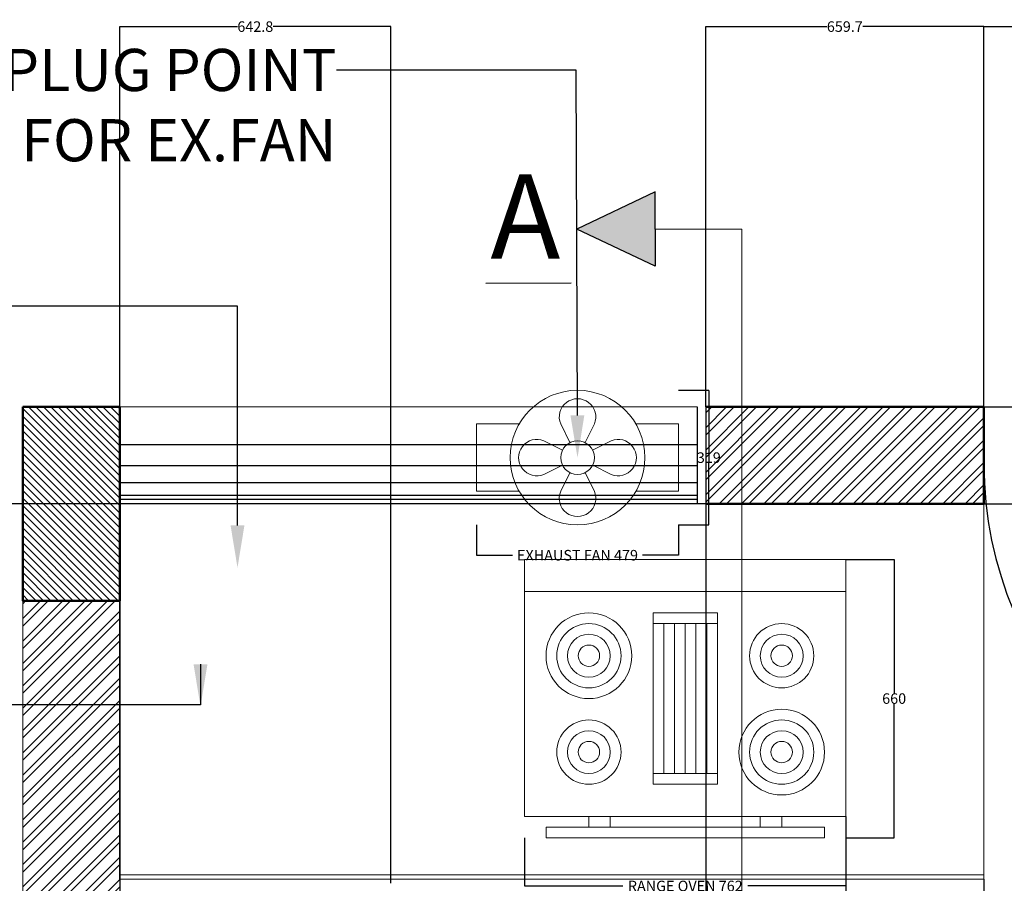
# Model space of a CAD drawing. Units: millimetres. Extents: x 1944 to 29915, y -10550 to 5909.
# Tile 8 of 24: x 6709 to 9044, y 3861 to 5909. Entities that reach past the tile are written whole.
import ezdxf
from ezdxf import colors
from ezdxf.entities.mleader import LeaderData, LeaderLine
from ezdxf.math import Vec2, Vec3

# ---------------------------------------------------------------- set-up
doc = ezdxf.new("R2010")
doc.units = ezdxf.units.MM
doc.header["$MEASUREMENT"] = 0
for name, color, linetype, lineweight in [('A-ANNO-DIMS', 2, 'Continuous', 18), ('A-ANNO-SYMB', 2, 'Continuous', 18), ('A-ANNO-TEXT', 7, 'Continuous', 25), ('A-DOOR', 4, 'Continuous', 25), ('A-EQPM', 6, 'Continuous', 18), ('A-FLOR-FIXT', 9, 'Continuous', 18), ('A-GLAZ', 4, 'Continuous', 25), ('A-WALL', 7, 'Continuous', 50), ('A-WALL-PATT', 8, 'Continuous', 18)]:
    doc.layers.add(name, color=color, linetype=linetype, lineweight=lineweight)
doc.styles.get("Standard").update_dxf_attribs({"font": 'arial.ttf'})
doc.dimstyles.get("Standard").update_dxf_attribs({"dimtxt": 25, "dimasz": 0.18, "dimexe": 0.18, "dimexo": 0.0625, "dimgap": 0.09, "dimtad": 0, "dimtih": 1, "dimtoh": 1, "dimdec": 0, "dimzin": 0, "dimdsep": 46, "dimtxsty": 'Standard', "dimcen": 0.09, "dimadec": 0, "dimazin": 0, "dimtfac": 1, "dimtdec": 0, "dimtofl": 0, "dimtmove": 0, "dimatfit": 3, "dimfxl": 1, "dimtolj": 1, "dimtzin": 0, "dimarcsym": 0})

# ---------------------------------------------------------------- blocks, each defined once
blk = doc.blocks.new('Range-Oven - 30 in top')
for p, q in [((0, -3), (30, -3)), ((12, -6), (18, -6)), ((13, -20), (13, -6)), ((14, -6), (14, -20)), ((15, -20), (15, -6)), ((16, -6), (16, -20)), ((17, -20), (17, -6)), ((18, -20), (12, -20)), ((6, -24), (6, -25)), ((8, -25), (8, -24)), ((22, -25), (22, -24)), ((24, -24), (24, -25))]:
    blk.add_line(p, q)
for points in [[(0, -24), (0, 0), (30, 0), (30, -24)], [(12, -21), (12, -5), (18, -5), (18, -21)], [(2, -26), (2, -25), (28, -25), (28, -26)]]:
    blk.add_lwpolyline(points, close=True)
for centre, radius in [((6, -9), 4), ((6, -9), 3), ((24, -9), 3), ((6, -9), 2), ((24, -9), 2), ((6, -9), 1), ((24, -9), 1), ((24, -18), 4), ((6, -18), 3), ((24, -18), 3), ((6, -18), 2), ((24, -18), 2), ((6, -18), 1), ((24, -18), 1)]:
    blk.add_circle(centre, radius)
blk = doc.blocks.new('Fan')
for p, q in [((0, 0), (0, 0.1)), ((0, 0.1), (0.1287, 0.1)), ((0.2776, 0.0448), (0.25, 0.1)), ((0.35, 0.1), (0.3225, 0.045)), ((0.473, 0.1), (0.6, 0.1)), ((0.6, 0.1), (0.6, 0)), ((0.2552, 0.0224), (0.2, 0.05)), ((0.3448, 0.0224), (0.4, 0.05)), ((0, -0.1), (0, 0)), ((0.6, 0), (0.6, -0.1)), ((0.2, -0.05), (0.255, -0.0225)), ((0.4, -0.05), (0.345, -0.0225)), ((0.2776, -0.0448), (0.25, -0.1)), ((0.35, -0.1), (0.3225, -0.045)), ((0.1278, -0.1), (0, -0.1)), ((0.6, -0.1), (0.4736, -0.1))]:
    blk.add_line(p, q)
blk.add_circle((0.3, 0), 0.05)
for centre, radius, start, end in [((0.3, 0), 0.2, 90, 180), ((0.3, 0), 0.2, 0, 90), ((0.3, 0.1208), 0.0542, 337.3801, 202.6199), ((0.1792, 0), 0.0542, 67.3801, 292.6199), ((0.4208, 0), 0.0542, 247.3801, 112.6199), ((0.3, 0), 0.2, 180, 270), ((0.3, 0), 0.2, 270, 0), ((0.3, -0.1208), 0.0542, 157.3801, 22.6199)]:
    blk.add_arc(centre, radius, start, end)
blk = doc.blocks.new('*U2')
for p, q in [((0, 0), (0, -6)), ((40, 0), (40, -6))]:
    blk.add_line(p, q)
blk.add_lwpolyline([(0, 0), (0, 40), (1.75, 40), (1.75, 0)], close=True)
blk.add_arc((0, 0), 40, 0, 90)
blk = doc.blocks.new('*D38')
at = {"layer": 'A-ANNO-DIMS', "color": 0, "lineweight": -2, "transparency": 16777216}
for p, q in [((7906, 3968.8), (7906, 3854.4)), ((8668, 3968.8), (8668, 3854.4)), ((7906.2, 3854.5), (8138.8, 3854.5)), ((8667.9, 3854.5), (8435.3, 3854.5))]:
    blk.add_line(p, q, dxfattribs=at)
at = {"layer": 'A-ANNO-DIMS', "color": 0, "transparency": 16777216}
for points in [[(7906.2, 3854.6), (7906.2, 3854.5), (7906, 3854.5)], [(8667.9, 3854.6), (8667.9, 3854.5), (8668, 3854.5)]]:
    blk.add_solid(points, dxfattribs=at)
at = {"layer": 'Defpoints', "color": 0, "transparency": 16777216}
for p in [(7906, 3968.8), (8668, 3968.8), (8668, 3854.5)]:
    blk.add_point(p, dxfattribs=at)
at = {"layer": 'A-ANNO-DIMS', "color": 0, "transparency": 16777216, "insert": (8287, 3854.5), "char_height": 25, "attachment_point": 5}
blk.add_mtext('\\A1;RANGE OVEN 762', dxfattribs=at)
blk = doc.blocks.new('*D39')
at = {"layer": 'A-ANNO-DIMS', "color": 0, "lineweight": -2, "transparency": 16777216}
for p, q in [((8668.1, 4629.2), (8782.5, 4629.2)), ((8782.3, 4629.1), (8782.3, 4311.9)), ((8782.3, 3969), (8782.3, 4286.2)), ((8668.1, 3968.8), (8782.5, 3968.8))]:
    blk.add_line(p, q, dxfattribs=at)
at = {"layer": 'A-ANNO-DIMS', "color": 0, "transparency": 16777216}
for points in [[(8782.3, 4629.1), (8782.4, 4629.1), (8782.3, 4629.2)], [(8782.3, 3969), (8782.4, 3969), (8782.3, 3968.8)]]:
    blk.add_solid(points, dxfattribs=at)
at = {"layer": 'Defpoints', "color": 0, "transparency": 16777216}
for p in [(8668, 4629.2), (8782.3, 4629.2), (8668, 3968.8)]:
    blk.add_point(p, dxfattribs=at)
at = {"layer": 'A-ANNO-DIMS', "color": 0, "transparency": 16777216, "insert": (8782.3, 4299), "char_height": 25, "attachment_point": 5}
blk.add_mtext('\\A1;660', dxfattribs=at)
blk = doc.blocks.new('*D44')
at = {"layer": 'A-ANNO-DIMS', "color": 0, "lineweight": -2, "transparency": 16777216}
for p, q in [((7792, 4710.8), (7792, 4638.8)), ((8271, 4710.8), (8271, 4638.8)), ((7792.2, 4639), (7877.3, 4639)), ((8270.8, 4639), (8185.7, 4639))]:
    blk.add_line(p, q, dxfattribs=at)
at = {"layer": 'A-ANNO-DIMS', "color": 0, "transparency": 16777216}
for points in [[(7792.2, 4639), (7792.2, 4638.9), (7792, 4639)], [(8270.8, 4639), (8270.8, 4638.9), (8271, 4639)]]:
    blk.add_solid(points, dxfattribs=at)
at = {"layer": 'Defpoints', "color": 0, "transparency": 16777216}
for p in [(7792, 4710.8), (8271, 4710.8), (8271, 4639)]:
    blk.add_point(p, dxfattribs=at)
at = {"layer": 'A-ANNO-DIMS', "color": 0, "transparency": 16777216, "insert": (8031.5, 4639), "char_height": 25, "attachment_point": 5}
blk.add_mtext('\\A1;EXHAUST FAN 479', dxfattribs=at)
blk = doc.blocks.new('*D45')
at = {"layer": 'A-ANNO-DIMS', "color": 0, "lineweight": -2, "transparency": 16777216}
for p, q in [((8271, 5030.1), (8343, 5030.1)), ((8342.8, 5030), (8342.8, 4883.3)), ((8342.8, 4711), (8342.8, 4857.6)), ((8271, 4710.8), (8343, 4710.8))]:
    blk.add_line(p, q, dxfattribs=at)
at = {"layer": 'A-ANNO-DIMS', "color": 0, "transparency": 16777216}
for points in [[(8342.8, 5030), (8342.9, 5030), (8342.8, 5030.1)], [(8342.8, 4711), (8342.9, 4711), (8342.8, 4710.8)]]:
    blk.add_solid(points, dxfattribs=at)
at = {"layer": 'Defpoints', "color": 0, "transparency": 16777216}
for p in [(8271, 5030.1), (8342.8, 5030.1), (8271, 4710.8)]:
    blk.add_point(p, dxfattribs=at)
at = {"layer": 'A-ANNO-DIMS', "color": 0, "transparency": 16777216, "insert": (8342.8, 4870.5), "char_height": 25, "attachment_point": 5}
blk.add_mtext('\\A1;319', dxfattribs=at)
blk = doc.blocks.new('*D46')
at = {"layer": 'A-ANNO-DIMS', "color": 0, "lineweight": -2, "transparency": 16777216}
for p, q in [((8335.5, 4990.9), (8335.5, 5892.9)), ((8335.7, 5892.8), (8623, 5892.8)), ((8995, 5892.8), (8707.7, 5892.8)), ((8995.2, 4990.9), (8995.2, 5892.9))]:
    blk.add_line(p, q, dxfattribs=at)
at = {"layer": 'A-ANNO-DIMS', "color": 0, "transparency": 16777216}
for points in [[(8335.7, 5892.8), (8335.7, 5892.7), (8335.5, 5892.8)], [(8995, 5892.8), (8995, 5892.7), (8995.2, 5892.8)]]:
    blk.add_solid(points, dxfattribs=at)
at = {"layer": 'Defpoints', "color": 0, "transparency": 16777216}
for p in [(8995.2, 5892.8), (8335.5, 4990.8), (8995.2, 4990.8)]:
    blk.add_point(p, dxfattribs=at)
at = {"layer": 'A-ANNO-DIMS', "color": 0, "transparency": 16777216, "insert": (8665.3, 5892.8), "char_height": 25, "attachment_point": 5}
blk.add_mtext('\\A1;659.7', dxfattribs=at)
blk = doc.blocks.new('*D47')
at = {"layer": 'A-ANNO-DIMS', "color": 0, "lineweight": -2, "transparency": 16777216}
for p, q in [((8995.2, 4990.9), (8995.2, 5892.9)), ((8995.4, 5892.8), (9417.6, 5892.8)), ((9895, 5892.8), (9472.9, 5892.8)), ((9895.2, 4990.9), (9895.2, 5892.9))]:
    blk.add_line(p, q, dxfattribs=at)
at = {"layer": 'A-ANNO-DIMS', "color": 0, "transparency": 16777216}
for points in [[(8995.4, 5892.8), (8995.4, 5892.7), (8995.2, 5892.8)], [(9895, 5892.8), (9895, 5892.7), (9895.2, 5892.8)]]:
    blk.add_solid(points, dxfattribs=at)
at = {"layer": 'Defpoints', "color": 0, "transparency": 16777216}
for p in [(9895.2, 5892.8), (8995.2, 4990.8), (9895.2, 4990.8)]:
    blk.add_point(p, dxfattribs=at)
at = {"layer": 'A-ANNO-DIMS', "color": 0, "transparency": 16777216, "insert": (9445.2, 5892.8), "char_height": 25, "attachment_point": 5}
blk.add_mtext('\\A1;900', dxfattribs=at)
blk = doc.blocks.new('*D49')
at = {"layer": 'A-ANNO-DIMS', "color": 0, "lineweight": -2, "transparency": 16777216}
for p, q in [((8335.5, 4760.8), (8335.5, -697.2)), ((6945.9, 4530.8), (6945.9, -697.2)), ((6946.1, -697), (7589.8, -697)), ((8335.3, -697), (7691.6, -697))]:
    blk.add_line(p, q, dxfattribs=at)
at = {"layer": 'A-ANNO-DIMS', "color": 0, "transparency": 16777216}
for points in [[(6946.1, -697), (6946.1, -697.1), (6945.9, -697)], [(8335.3, -697), (8335.3, -697.1), (8335.5, -697)]]:
    blk.add_solid(points, dxfattribs=at)
at = {"layer": 'Defpoints', "color": 0, "transparency": 16777216}
for p in [(8335.5, 4760.8), (6945.9, 4530.8), (8335.5, -697)]:
    blk.add_point(p, dxfattribs=at)
at = {"layer": 'A-ANNO-DIMS', "color": 0, "transparency": 16777216, "insert": (7640.7, -697), "char_height": 25, "attachment_point": 5}
blk.add_mtext('\\A1;1389.5', dxfattribs=at)
blk = doc.blocks.new('*D55')
at = {"layer": 'A-ANNO-DIMS', "color": 0, "lineweight": -2, "transparency": 16777216}
for p, q in [((8995.3, 4990.8), (11007.7, 4990.8)), ((11007.5, 4990.7), (11007.5, 4888.7)), ((11007.5, 4761), (11007.5, 4863)), ((8995.3, 4760.8), (11007.7, 4760.8))]:
    blk.add_line(p, q, dxfattribs=at)
at = {"layer": 'A-ANNO-DIMS', "color": 0, "transparency": 16777216}
for points in [[(11007.5, 4990.7), (11007.5, 4990.7), (11007.5, 4990.8)], [(11007.5, 4761), (11007.5, 4761), (11007.5, 4760.8)]]:
    blk.add_solid(points, dxfattribs=at)
at = {"layer": 'Defpoints', "color": 0, "transparency": 16777216}
for p in [(8995.2, 4990.8), (8995.2, 4760.8), (11007.5, 4760.8)]:
    blk.add_point(p, dxfattribs=at)
at = {"layer": 'A-ANNO-DIMS', "color": 0, "transparency": 16777216, "insert": (11007.5, 4875.8), "char_height": 25, "attachment_point": 5}
blk.add_mtext('\\A1;230', dxfattribs=at)
blk = doc.blocks.new('*D57')
at = {"layer": 'A-ANNO-DIMS', "color": 0, "lineweight": -2, "transparency": 16777216}
for p, q in [((8995.2, 4760.8), (5803.8, 4760.8)), ((5804, 4760.7), (5804, 2520.7)), ((5804, 255), (5804, 2495)), ((8999.6, 254.8), (5803.8, 254.8))]:
    blk.add_line(p, q, dxfattribs=at)
at = {"layer": 'A-ANNO-DIMS', "color": 0, "transparency": 16777216}
for points in [[(5804, 4760.7), (5804, 4760.7), (5804, 4760.8)], [(5804, 255), (5804, 255), (5804, 254.8)]]:
    blk.add_solid(points, dxfattribs=at)
at = {"layer": 'Defpoints', "color": 0, "transparency": 16777216}
for p in [(8995.2, 4760.8), (5804, 254.8), (8999.6, 254.8)]:
    blk.add_point(p, dxfattribs=at)
at = {"layer": 'A-ANNO-DIMS', "color": 0, "transparency": 16777216, "insert": (5804, 2507.8), "char_height": 25, "attachment_point": 5}
blk.add_mtext('\\A1;4506', dxfattribs=at)
blk = doc.blocks.new('*D58')
at = {"layer": 'A-ANNO-DIMS', "color": 0, "lineweight": -2, "transparency": 16777216}
for p, q in [((6945.9, 3870.9), (6945.9, 5892.9)), ((6946.1, 5892.8), (7225, 5892.8)), ((7588.6, 5892.8), (7309.7, 5892.8)), ((7588.8, 3860.9), (7588.8, 5892.9))]:
    blk.add_line(p, q, dxfattribs=at)
at = {"layer": 'A-ANNO-DIMS', "color": 0, "transparency": 16777216}
for points in [[(6946.1, 5892.8), (6946.1, 5892.7), (6945.9, 5892.8)], [(7588.6, 5892.8), (7588.6, 5892.7), (7588.8, 5892.8)]]:
    blk.add_solid(points, dxfattribs=at)
at = {"layer": 'Defpoints', "color": 0, "transparency": 16777216}
for p in [(7588.8, 5892.8), (6945.9, 3870.8), (7588.8, 3860.8)]:
    blk.add_point(p, dxfattribs=at)
at = {"layer": 'A-ANNO-DIMS', "color": 0, "transparency": 16777216, "insert": (7267.4, 5892.8), "char_height": 25, "attachment_point": 5}
blk.add_mtext('\\A1;642.8', dxfattribs=at)
blk = doc.blocks.new('*D59')
at = {"layer": 'A-ANNO-DIMS', "color": 0, "lineweight": -2, "transparency": 16777216}
for p, q in [((8668, 4019.6), (8668, -697.2)), ((8995.2, 3870.8), (8995.2, -697.2)), ((8668.2, -697), (8789.5, -697)), ((8995, -697), (8873.8, -697))]:
    blk.add_line(p, q, dxfattribs=at)
at = {"layer": 'A-ANNO-DIMS', "color": 0, "transparency": 16777216}
for points in [[(8668.2, -697), (8668.2, -697.1), (8668, -697)], [(8995, -697), (8995, -697.1), (8995.2, -697)]]:
    blk.add_solid(points, dxfattribs=at)
at = {"layer": 'Defpoints', "color": 0, "transparency": 16777216}
for p in [(8668, 4019.6), (8995.2, 3870.8), (8995.2, -697)]:
    blk.add_point(p, dxfattribs=at)
at = {"layer": 'A-ANNO-DIMS', "color": 0, "transparency": 16777216, "insert": (8831.6, -697), "char_height": 25, "attachment_point": 5}
blk.add_mtext('\\A1;327.2', dxfattribs=at)

msp = doc.modelspace()

# ---------------------------------------------------------------- hatches: boundary and pattern name
at = {"layer": 'A-ANNO-SYMB'}
h = msp.add_hatch(color=256, dxfattribs=at)
h.dxf.hatch_style = 1
h.paths.add_polyline_path([(8215.358, 5500.519), (8029.821, 5412.489), (8215.358, 5324.458), (8215.358, 5412.489)])
at = {"layer": 'A-WALL-PATT'}
h = msp.add_hatch(dxfattribs=at)
h.set_pattern_fill('ANSI31', color=256, scale=100, angle=90)
h.paths.add_polyline_path([(6715.942, 4530.837), (6945.942, 4530.837), (6945.942, 4990.837), (6715.942, 4990.837)])
h = msp.add_hatch(dxfattribs=at)
h.set_pattern_fill('ANSI32', color=256, scale=100)
h.paths.add_polyline_path([(8995.217, 4760.837), (8995.217, 4990.837), (8335.477, 4990.837), (8335.477, 4760.837)])
h = msp.add_hatch(dxfattribs=at)
h.set_pattern_fill('ANSI32', color=256, scale=100)
h.paths.add_polyline_path([(6945.942, 4530.837), (6715.942, 4530.837), (6715.942, 490.837), (6945.942, 490.837)])

# ---------------------------------------------------------------- linework, layer by layer
at = {"layer": 'A-ANNO-SYMB'}
msp.add_line((8420.942, -176.269), (8420.942, 5412.489), dxfattribs=at)
at = {"layer": 'A-DOOR'}
msp.add_line((8995.217, 4990.837), (9895.217, 4990.837), dxfattribs=at)
at = {"layer": 'A-FLOR-FIXT'}
for p, q in [((8420.942, 5412.489), (8215.358, 5412.489)), ((8995.217, 4760.837), (8995.217, 3860.837)), ((8995.217, 3880.837), (6945.942, 3880.837)), ((8995.217, 3870.837), (6945.942, 3870.837))]:
    msp.add_line(p, q, dxfattribs=at)
for points in [[(8995.217, 30.837), (6715.942, 30.837), (6715.942, 4990.837), (8315.477, 4990.837)], [(9000.245, 260.837), (6945.942, 260.837), (6945.942, 4760.837), (8315.477, 4760.837)]]:
    msp.add_lwpolyline(points, dxfattribs=at)
at = {"layer": 'A-GLAZ'}
for p, q in [((8215.358, 5500.519), (8029.821, 5412.489)), ((8215.358, 5412.489), (8215.358, 5500.519)), ((8215.358, 5324.458), (8029.821, 5412.489)), ((8215.358, 5412.489), (8215.358, 5324.458)), ((7814.164, 5283.975), (8016.766, 5284.993)), ((8315.477, 4990.837), (8315.477, 4760.837)), ((8335.477, 4990.837), (8335.477, 4760.837)), ((8315.477, 4900.837), (6945.942, 4900.837)), ((8315.477, 4850.837), (6945.942, 4850.837)), ((8315.477, 4810.837), (6945.942, 4810.837)), ((8315.477, 4780.837), (6945.942, 4780.837)), ((8315.477, 4770.837), (6945.942, 4770.837)), ((8315.477, 4760.837), (6945.942, 4760.837))]:
    msp.add_line(p, q, dxfattribs=at)
at = {"layer": 'A-WALL'}
msp.add_line((8995.217, 4760.837), (8995.217, 4990.837), dxfattribs=at)
msp.add_lwpolyline([(6715.942, 4990.837), (6945.942, 4990.837), (6945.942, 4530.837), (6715.942, 4530.837)], close=True, dxfattribs=at)
for points in [[(8335.477, 4990.837), (8995.217, 4990.837)], [(8335.477, 4760.837), (8995.217, 4760.837)]]:
    msp.add_lwpolyline(points, dxfattribs=at)

# ---------------------------------------------------------------- block references
at = {"layer": 'A-DOOR', "xscale": 22.5, "yscale": 22.5, "zscale": 22.5, "rotation": 180}
msp.add_blockref('*U2', (9895.217, 4855.837), dxfattribs=at)
at = {"layer": 'A-EQPM', "xscale": 798.2945614878786, "yscale": 798.2945614878786, "zscale": 798.2945614878786}
msp.add_blockref('Fan', (7792.008, 4870.48), dxfattribs=at)
at = {"layer": 'A-FLOR-FIXT', "xscale": 25.4, "yscale": 25.4, "zscale": 25.4}
msp.add_blockref('Range-Oven - 30 in top', (7906.038, 4629.243), dxfattribs=at)

# ---------------------------------------------------------------- texts
at = {"layer": 'A-ANNO-TEXT'}
msp.add_text('A', height=200, dxfattribs=at).set_placement((7824.811, 5342.033))

# ---------------------------------------------------------------- dimensions: what is measured, and where the dimension line sits
at = {"layer": 'A-ANNO-DIMS'}
for base, p1, p2, override, picture, middle in [((7588.787, 5892.769), (6945.942, 3870.837), (7588.787, 3860.837), {"dimdec": 1, "dimlfac": 1, "dimrnd": 0, "dimzin": 0, "dimdsep": 46, "dimlunit": 2}, '*D58', (7267.365, 5892.769)), ((8995.217, 5892.769), (8335.477, 4990.837), (8995.217, 4990.837), {"dimdec": 1, "dimlfac": 1, "dimrnd": 0, "dimzin": 0, "dimdsep": 46, "dimlunit": 2}, '*D46', (8665.347, 5892.769)), ((9895.217, 5892.769), (8995.217, 4990.837), (9895.217, 4990.837), {"dimdec": 0, "dimlfac": 1, "dimrnd": 0, "dimzin": 0, "dimdsep": 46, "dimlunit": 2}, '*D47', (9445.217, 5892.769)), ((8335.477, -697.033), (6945.942, 4530.837), (8335.477, 4760.837), {"dimdec": 1, "dimlfac": 1, "dimrnd": 0, "dimzin": 0, "dimdsep": 46, "dimlunit": 2}, '*D49', (7640.71, -697.033)), ((8995.217, -697.033), (8668.038, 4019.643), (8995.217, 3870.837), {"dimdec": 1, "dimlfac": 1, "dimrnd": 0, "dimzin": 0, "dimdsep": 46, "dimlunit": 2}, '*D59', (8831.628, -697.033))]:
    dim = msp.add_linear_dim(base=base, p1=p1, p2=p2, dimstyle='Standard', override=override, dxfattribs=at)
    dim.commit()
    dim.dimension.update_dxf_attribs({"geometry": picture, "text_midpoint": middle})
for base, p1, p2, override, picture, middle in [((8342.833, 5030.139), (8270.986, 4710.821), (8270.986, 5030.139), {"dimdec": 0, "dimrnd": 0, "dimzin": 0, "dimlunit": 2}, '*D45', (8342.833, 4870.48)), ((11007.504, 4760.837), (8995.217, 4990.837), (8995.217, 4760.837), {"dimdec": 0, "dimlfac": 1, "dimrnd": 0, "dimzin": 0, "dimdsep": 46, "dimlunit": 2}, '*D55', (11007.504, 4875.837)), ((5803.984, 254.791), (8995.217, 4760.837), (8999.621, 254.791), {"dimdec": 0, "dimlfac": 1, "dimrnd": 0, "dimzin": 0, "dimdsep": 46, "dimlunit": 2}, '*D57', (5803.984, 2507.814)), ((8782.338, 4629.243), (8668.038, 3968.843), (8668.038, 4629.243), {"dimdec": 0, "dimrnd": 0, "dimzin": 0, "dimlunit": 2}, '*D39', (8782.338, 4299.043))]:
    dim = msp.add_linear_dim(base=base, p1=p1, p2=p2, angle=90, dimstyle='Standard', override=override, dxfattribs=at)
    dim.commit()
    dim.dimension.update_dxf_attribs({"geometry": picture, "text_midpoint": middle})
for base, p1, p2, text, picture, middle in [((8270.986, 4638.975), (7792.008, 4710.821), (8270.986, 4710.821), 'EXHAUST FAN <>', '*D44', (8031.497, 4638.975)), ((8668.038, 3854.543), (7906.038, 3968.843), (8668.038, 3968.843), 'RANGE OVEN <>', '*D38', (8287.038, 3854.543))]:
    dim = msp.add_linear_dim(base=base, p1=p1, p2=p2, text=text, dimstyle='Standard', override={"dimdec": 0, "dimrnd": 0, "dimzin": 0, "dimlunit": 2}, dxfattribs=at)
    dim.commit()
    dim.dimension.update_dxf_attribs({"geometry": picture, "text_midpoint": middle})

# ---------------------------------------------------------------- leaders
at = {"layer": 'A-ANNO-TEXT'}
ml = msp.add_multileader_mtext('Standard', dxfattribs=at)
ml.set_content('6 AMP PLUG POINT\\PFOR EX.FAN ', color=256)
ml.set_leader_properties()
ml.build(insert=Vec2(0, 0))
ml.multileader.update_dxf_attribs({"dogleg_length": 568.936, "arrow_head_size": 100})
ctx = ml.context
ctx.base_point, ctx.char_height, ctx.arrow_head_size, ctx.landing_gap_size, ctx.plane_origin = Vec3(6163.428, 5789.061), 100, 100, 0.09, Vec3(7359.519, 5416.773)
ctx.text_align_type = 2
notes = []
notes.append((ctx, [(0, (1, 1, 0), (8028.655, 5789.061), (-1, 0), 568.936, [(0, [(8031.498, 4870.48), (8028.655, 5789.061)], 0, [])])]))
ctx.mtext.insert, ctx.mtext.alignment, ctx.mtext.flow_direction = Vec3(7459.63, 5839.914), 3, 5
ml = msp.add_multileader_mtext('Standard', dxfattribs=at)
ml.set_content('IIEAT PROOF COUNTER', color=256)
ml.set_leader_properties()
ml.build(insert=Vec2(0, 0))
ml.multileader.update_dxf_attribs({"dogleg_length": 568.936, "arrow_head_size": 100})
ctx = ml.context
ctx.base_point, ctx.char_height, ctx.arrow_head_size, ctx.landing_gap_size, ctx.plane_origin = Vec3(4680.871, 5230.05), 100, 100, 0.09, Vec3(6849.578, 5230.05)
ctx.text_align_type = 2
notes.append((ctx, [(0, (1, 1, 0), (6849.578, 5230.05), (-1, 0), 568.936, [(0, [(7225.221, 4609.585), (7225.221, 5230.05)], 0, [])])]))
ctx.mtext.insert, ctx.mtext.alignment, ctx.mtext.flow_direction = Vec3(6280.552, 5280.903), 3, 5
ml = msp.add_multileader_mtext('Standard', dxfattribs=at)
ml.set_content('CHOPPING COUNTER', color=256)
ml.set_leader_properties()
ml.build(insert=Vec2(0, 0))
ml.multileader.update_dxf_attribs({"dogleg_length": 568.936, "arrow_head_size": 100})
ctx = ml.context
ctx.base_point, ctx.char_height, ctx.arrow_head_size, ctx.landing_gap_size, ctx.plane_origin = Vec3(4308.291, 4284.103), 100, 100, 0.09, Vec3(6343.369, 4284.103)
ctx.text_align_type = 2
notes.append((ctx, [(0, (1, 1, 0), (6343.369, 4284.103), (-1, 0), 568.936, [(0, [(7137.476, 4280.213), (7137.476, 4284.103)], 0, [])])]))
ctx.mtext.insert, ctx.mtext.alignment, ctx.mtext.flow_direction = Vec3(5774.343, 4334.955), 3, 5
for ctx, leaders in notes:
    for number, flags, end, landing, length, lines in leaders:
        leader = LeaderData()
        leader.index, (leader.has_last_leader_line, leader.has_dogleg_vector, leader.attachment_direction) = number, flags
        leader.last_leader_point, leader.dogleg_vector, leader.dogleg_length = Vec3(end), Vec3(landing), length
        for number, points, colour, breaks in lines:
            line = LeaderLine()
            line.index, line.vertices, line.color, line.breaks = number, Vec3.list(points), colors.encode_raw_color(colour), breaks
            leader.lines.append(line)
        ctx.leaders.append(leader)

doc.saveas('drawing.dxf')
